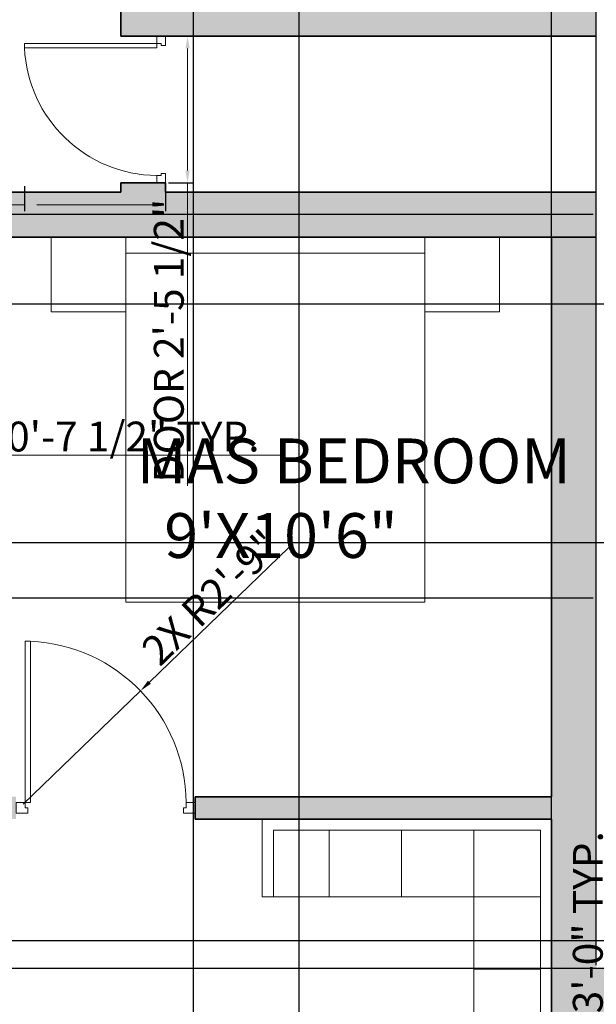
# Model space of a CAD drawing. Units: inches. Extents: x 2696 to 3240, y 1564 to 2310.
# Tile 52 of 76: x 2850 to 2966, y 1982 to 2180. Entities that reach past the tile are written whole.
import ezdxf

# ---------------------------------------------------------------- set-up
doc = ezdxf.new("R2010")
doc.units = ezdxf.units.IN
doc.linetypes.add('ACAD_ISO02W100', pattern=[15, 12, -3])
for name, color, linetype, lineweight in [('A-ANNO-DIMS', 3, 'Continuous', 18), ('A-AREA-IDEN', 7, 'Continuous', 18), ('A-DOOR', 4, 'Continuous', 18), ('A-FURN', 251, 'Continuous', 13), ('A-WALL', 7, 'Continuous', 35), ('A-WALL-OVHD', 7, 'ACAD_ISO02W100', 18), ('A-WALL-PATT', 9, 'Continuous', 13)]:
    doc.layers.add(name, color=color, linetype=linetype, lineweight=lineweight)
doc.styles.add('TIMES NEW', font='times.ttf')
doc.styles.add('YQ_DIM', font='SUPEROS.SHX', dxfattribs={"width": 0.8, "bigfont": 'HZDX.SHX'})
doc.dimstyles.new('Siddhuu', dxfattribs={"dimtxt": 6, "dimasz": 2.5, "dimexe": 1.25, "dimexo": 0.625, "dimtad": 1, "dimdec": 1, "dimlunit": 4, "dimtxsty": 'TIMES NEW', "dimcen": 2.5, "dimclrd": 256, "dimclre": 1, "dimclrt": 7, "dimadec": 0, "dimazin": 0, "dimtfac": 1, "dimtdec": 1, "dimtmove": 0, "dimatfit": 3, "dimfxl": 1, "dimtolj": 1, "dimlwd": -1, "dimarcsym": 0})

# ---------------------------------------------------------------- blocks, each defined once
blk = doc.blocks.new('DR_D01')
for p, q in [((-0.45, 0.93), (-0.42, 0.93)), ((-0.45, 0.03), (-0.45, 0.93)), ((-0.42, 0.03), (-0.42, 0.93)), ((-0.5, 0.03), (-0.42, 0.03)), ((-0.5, 0.03), (-0.5, -0.03)), ((-0.45, 0.03), (-0.45, 0)), ((-0.45, 0), (-0.435, 0)), ((-0.435, 0), (-0.435, -0.03)), ((0.435, 0), (0.435, -0.03)), ((0.45, 0), (0.435, 0)), ((0.45, 0.03), (0.45, 0)), ((0.5, 0.03), (0.45, 0.03)), ((0.5, -0.03), (0.5, 0.03)), ((-0.435, -0.03), (-0.5, -0.03)), ((0.435, -0.03), (0.5, -0.03))]:
    blk.add_line(p, q)
blk.add_arc((-0.4602, 0.0206), 0.9103, 0.5915, 87.4664)
blk = doc.blocks.new('BED-DOUBLE-WITH-NIGHTSTANDS')
for points in [[(0, 75.13), (0, 90.16), (15.03, 90.16), (15.03, 75.13)], [(3.28, 15.03), (3.28, 75.13), (73.4, 75.13), (73.4, 15.03)], [(0, 15.03), (0, 0), (15.03, 0), (15.03, 15.03)]]:
    blk.add_lwpolyline(points, close=True)
blk = doc.blocks.new('SOFA-SECTIONAL')
for p, q in [((0, 43.61), (0, 59.26)), ((0, 59.26), (58.14, 59.26)), ((58.14, 59.26), (58.14, 0)), ((2.24, 43.61), (2.24, 57.02)), ((2.24, 57.02), (55.9, 57.02)), ((13.42, 57.02), (13.42, 43.61)), ((27.95, 57.02), (27.95, 43.61)), ((42.49, 57.02), (42.49, 0)), ((55.9, 57.02), (55.9, 2.24)), ((0, 43.61), (55.9, 43.61)), ((42.49, 29.07), (55.9, 29.07)), ((42.49, 14.54), (55.9, 14.54)), ((55.9, 2.24), (42.49, 2.24)), ((58.14, 0), (42.49, 0))]:
    blk.add_line(p, q)
blk = doc.blocks.new('*D28')
at = {"layer": 'A-ANNO-DIMS', "color": 1, "lineweight": -2, "transparency": 16777216}
for p, q in [((2879.74, 2176.6), (2884.79, 2176.6)), ((2879.74, 2147.07), (2884.79, 2147.07))]:
    blk.add_line(p, q, dxfattribs=at)
at = {"layer": 'A-ANNO-DIMS', "transparency": 16777216}
for p, q in [((2883.54, 2174.1), (2883.54, 2149.57)), ((2883.54, 2147.07), (2883.54, 2086.19))]:
    blk.add_line(p, q, dxfattribs=at)
for points in [[(2883.12, 2174.1), (2883.96, 2174.1), (2883.54, 2176.6)], [(2883.12, 2149.57), (2883.96, 2149.57), (2883.54, 2147.07)]]:
    blk.add_solid(points, dxfattribs=at)
at = {"layer": 'Defpoints', "color": 0, "transparency": 16777216}
for p in [(2879.11, 2176.6), (2879.11, 2147.07), (2883.54, 2147.07)]:
    blk.add_point(p, dxfattribs=at)
at = {"layer": 'A-ANNO-DIMS', "color": 7, "transparency": 16777216, "insert": (2879.77, 2115.38), "char_height": 6, "attachment_point": 5, "rotation": 90, "style": 'TIMES NEW'}
blk.add_mtext('\\A1;DOOR 2\'-5 1/2"', dxfattribs=at)
blk = doc.blocks.new('*D29')
at = {"layer": 'A-ANNO-DIMS', "color": 1, "lineweight": -2, "transparency": 16777216}
for p, q in [((2850.76, 2146.45), (2850.76, 2141.39)), ((2879.11, 2146.45), (2879.11, 2141.39))]:
    blk.add_line(p, q, dxfattribs=at)
at = {"layer": 'A-ANNO-DIMS', "transparency": 16777216}
for p, q in [((2850.76, 2142.64), (2817.24, 2142.64)), ((2876.61, 2142.64), (2853.26, 2142.64))]:
    blk.add_line(p, q, dxfattribs=at)
for points in [[(2853.26, 2143.06), (2853.26, 2142.23), (2850.76, 2142.64)], [(2876.61, 2143.06), (2876.61, 2142.23), (2879.11, 2142.64)]]:
    blk.add_solid(points, dxfattribs=at)
at = {"layer": 'Defpoints', "color": 0, "transparency": 16777216}
for p in [(2850.76, 2147.07), (2879.11, 2147.07), (2850.76, 2142.64)]:
    blk.add_point(p, dxfattribs=at)
at = {"layer": 'A-ANNO-DIMS', "color": 7, "transparency": 16777216, "insert": (2832.75, 2146.41), "char_height": 6, "attachment_point": 5, "style": 'TIMES NEW'}
blk.add_mtext('\\A1;2\'-4 1/2"', dxfattribs=at)
blk = doc.blocks.new('*D30')
at = {"layer": 'A-ANNO-DIMS', "transparency": 16777216}
for p, q in [((2967.69, 1950.58), (2967.69, 2019.05)), ((2967.69, 1917.08), (2967.69, 1948.08))]:
    blk.add_line(p, q, dxfattribs=at)
at = {"layer": 'A-ANNO-DIMS', "color": 1, "lineweight": -2, "transparency": 16777216}
for p, q in [((2962.91, 1950.58), (2968.94, 1950.58)), ((2962.91, 1914.58), (2968.94, 1914.58))]:
    blk.add_line(p, q, dxfattribs=at)
at = {"layer": 'A-ANNO-DIMS', "transparency": 16777216}
for points in [[(2967.27, 1948.08), (2968.11, 1948.08), (2967.69, 1950.58)], [(2967.27, 1917.08), (2968.11, 1917.08), (2967.69, 1914.58)]]:
    blk.add_solid(points, dxfattribs=at)
at = {"layer": 'Defpoints', "color": 0, "transparency": 16777216}
for p in [(2962.29, 1950.58), (2967.69, 1950.58), (2962.29, 1914.58)]:
    blk.add_point(p, dxfattribs=at)
at = {"layer": 'A-ANNO-DIMS', "color": 7, "transparency": 16777216, "insert": (2964, 1986.06), "char_height": 6, "attachment_point": 5, "rotation": 90, "style": 'TIMES NEW'}
blk.add_mtext('\\A1;DOOR 3\'-0" TYP.', dxfattribs=at)
blk = doc.blocks.new('*D40')
at = {"layer": 'A-ANNO-DIMS', "color": 1, "lineweight": -2, "transparency": 16777216}
for p, q in [((2777.27, 2091.83), (2777.27, 2093.58)), ((2784.76, 2091.83), (2784.76, 2093.58))]:
    blk.add_line(p, q, dxfattribs=at)
at = {"layer": 'A-ANNO-DIMS', "transparency": 16777216}
for p, q in [((2779.77, 2092.33), (2782.26, 2092.33)), ((2784.76, 2092.33), (2902.46, 2092.33))]:
    blk.add_line(p, q, dxfattribs=at)
for points in [[(2779.77, 2092.74), (2779.77, 2091.91), (2777.27, 2092.33)], [(2782.26, 2092.74), (2782.26, 2091.91), (2784.76, 2092.33)]]:
    blk.add_solid(points, dxfattribs=at)
at = {"layer": 'Defpoints', "color": 0, "transparency": 16777216}
for p in [(2784.76, 2092.33), (2777.27, 2091.2), (2784.76, 2091.2)]:
    blk.add_point(p, dxfattribs=at)
at = {"layer": 'A-ANNO-DIMS', "color": 7, "transparency": 16777216, "insert": (2844.86, 2096.09), "char_height": 6, "attachment_point": 5, "style": 'TIMES NEW'}
blk.add_mtext('\\A1;BATH FITTING 0\'-7 1/2" TYP.', dxfattribs=at)
blk = doc.blocks.new('*D57')
at = {"layer": 'A-ANNO-DIMS', "color": 1, "lineweight": -2, "transparency": 16777216}
for p, q in [((2754.61, 2018.58), (2754.61, 1568.95)), ((2956.71, 2018.58), (2956.71, 1568.95))]:
    blk.add_line(p, q, dxfattribs=at)
at = {"layer": 'A-ANNO-DIMS', "transparency": 16777216}
blk.add_line((2757.11, 1570.2), (2954.21, 1570.2), dxfattribs=at)
for points in [[(2757.11, 1570.62), (2757.11, 1569.78), (2754.61, 1570.2)], [(2954.21, 1570.62), (2954.21, 1569.78), (2956.71, 1570.2)]]:
    blk.add_solid(points, dxfattribs=at)
at = {"layer": 'Defpoints', "color": 0, "transparency": 16777216}
for p in [(2754.61, 2019.2), (2956.71, 2019.2), (2956.71, 1570.2)]:
    blk.add_point(p, dxfattribs=at)
at = {"layer": 'A-ANNO-DIMS', "color": 7, "transparency": 16777216, "insert": (2855.66, 1573.88), "char_height": 6, "attachment_point": 5, "style": 'TIMES NEW'}
blk.add_mtext('\\A1;16\'-10"', dxfattribs=at)
blk = doc.blocks.new('*D59')
at = {"layer": 'A-ANNO-DIMS', "color": 1, "lineweight": -2, "transparency": 16777216}
for p, q in [((2884.71, 1740.83), (2884.71, 2298.45)), ((2956.71, 1740.83), (2956.71, 2298.45))]:
    blk.add_line(p, q, dxfattribs=at)
at = {"layer": 'A-ANNO-DIMS', "transparency": 16777216}
blk.add_line((2887.21, 2297.2), (2954.21, 2297.2), dxfattribs=at)
for points in [[(2887.21, 2297.62), (2887.21, 2296.78), (2884.71, 2297.2)], [(2954.21, 2297.62), (2954.21, 2296.78), (2956.71, 2297.2)]]:
    blk.add_solid(points, dxfattribs=at)
at = {"layer": 'Defpoints', "color": 0, "transparency": 16777216}
for p in [(2956.71, 2297.2), (2884.71, 1740.2), (2956.71, 1740.2)]:
    blk.add_point(p, dxfattribs=at)
at = {"layer": 'A-ANNO-DIMS', "color": 7, "transparency": 16777216, "insert": (2920.71, 2300.88), "char_height": 6, "attachment_point": 5, "style": 'TIMES NEW'}
blk.add_mtext('\\A1;6\'-0"', dxfattribs=at)
blk = doc.blocks.new('*D61')
at = {"layer": 'A-ANNO-DIMS', "color": 1, "lineweight": -2, "transparency": 16777216}
for p, q in [((2965.71, 2141.33), (2965.71, 2298.45)), ((3044.3, 2141.33), (3044.3, 2298.45))]:
    blk.add_line(p, q, dxfattribs=at)
at = {"layer": 'A-ANNO-DIMS', "transparency": 16777216}
blk.add_line((2968.21, 2297.2), (3041.8, 2297.2), dxfattribs=at)
for points in [[(2968.21, 2297.62), (2968.21, 2296.78), (2965.71, 2297.2)], [(3041.8, 2297.62), (3041.8, 2296.78), (3044.3, 2297.2)]]:
    blk.add_solid(points, dxfattribs=at)
at = {"layer": 'Defpoints', "color": 0, "transparency": 16777216}
for p in [(3044.3, 2297.2), (2965.71, 2140.7), (3044.3, 2140.7)]:
    blk.add_point(p, dxfattribs=at)
at = {"layer": 'A-ANNO-DIMS', "color": 7, "transparency": 16777216, "insert": (3005.01, 2300.96), "char_height": 6, "attachment_point": 5, "style": 'TIMES NEW'}
blk.add_mtext('\\A1;6\'-6 1/2"', dxfattribs=at)
blk = doc.blocks.new('*D62')
at = {"layer": 'A-ANNO-DIMS', "color": 1, "lineweight": -2, "transparency": 16777216}
for p, q in [((2965.08, 2140.7), (2709.36, 2140.7)), ((2965.08, 2063.59), (2709.36, 2063.59))]:
    blk.add_line(p, q, dxfattribs=at)
at = {"layer": 'A-ANNO-DIMS', "transparency": 16777216}
blk.add_line((2710.61, 2066.09), (2710.61, 2138.2), dxfattribs=at)
for points in [[(2710.19, 2138.2), (2711.03, 2138.2), (2710.61, 2140.7)], [(2710.19, 2066.09), (2711.03, 2066.09), (2710.61, 2063.59)]]:
    blk.add_solid(points, dxfattribs=at)
at = {"layer": 'Defpoints', "color": 0, "transparency": 16777216}
for p in [(2710.61, 2140.7), (2965.71, 2140.7), (2965.71, 2063.59)]:
    blk.add_point(p, dxfattribs=at)
at = {"layer": 'A-ANNO-DIMS', "color": 7, "transparency": 16777216, "insert": (2706.93, 2102.15), "char_height": 6, "attachment_point": 5, "rotation": 90, "style": 'TIMES NEW'}
blk.add_mtext('\\A1;6\'-5"', dxfattribs=at)
blk = doc.blocks.new('*D63')
at = {"layer": 'A-ANNO-DIMS', "color": 1, "lineweight": -2, "transparency": 16777216}
for p, q in [((2965.71, 1989.83), (2965.71, 2298.45)), ((3069.21, 1989.83), (3069.21, 2298.45))]:
    blk.add_line(p, q, dxfattribs=at)
at = {"layer": 'A-ANNO-DIMS', "transparency": 16777216}
blk.add_line((2968.21, 2297.2), (3066.71, 2297.2), dxfattribs=at)
for points in [[(2968.21, 2297.62), (2968.21, 2296.78), (2965.71, 2297.2)], [(3066.71, 2297.62), (3066.71, 2296.78), (3069.21, 2297.2)]]:
    blk.add_solid(points, dxfattribs=at)
at = {"layer": 'Defpoints', "color": 0, "transparency": 16777216}
for p in [(3069.21, 2297.2), (2965.71, 1989.2), (3069.21, 1989.2)]:
    blk.add_point(p, dxfattribs=at)
at = {"layer": 'A-ANNO-DIMS', "color": 7, "transparency": 16777216, "insert": (3017.46, 2300.96), "char_height": 6, "attachment_point": 5, "style": 'TIMES NEW'}
blk.add_mtext('\\A1;8\'-7 1/2"', dxfattribs=at)
blk = doc.blocks.new('*D64')
at = {"layer": 'A-ANNO-DIMS', "color": 1, "lineweight": -2, "transparency": 16777216}
for p, q in [((3073.08, 2206.7), (2709.36, 2206.7)), ((3068.58, 1989.2), (2709.36, 1989.2))]:
    blk.add_line(p, q, dxfattribs=at)
at = {"layer": 'A-ANNO-DIMS', "transparency": 16777216}
blk.add_line((2710.61, 1991.7), (2710.61, 2204.2), dxfattribs=at)
for points in [[(2710.19, 2204.2), (2711.03, 2204.2), (2710.61, 2206.7)], [(2710.19, 1991.7), (2711.03, 1991.7), (2710.61, 1989.2)]]:
    blk.add_solid(points, dxfattribs=at)
at = {"layer": 'Defpoints', "color": 0, "transparency": 16777216}
for p in [(2710.61, 2206.7), (3073.71, 2206.7), (3069.21, 1989.2)]:
    blk.add_point(p, dxfattribs=at)
at = {"layer": 'A-ANNO-DIMS', "color": 7, "transparency": 16777216, "insert": (2706.85, 2097.95), "char_height": 6, "attachment_point": 5, "rotation": 90, "style": 'TIMES NEW'}
blk.add_mtext('\\A1;18\'-1 1/2"', dxfattribs=at)
blk = doc.blocks.new('*D66')
at = {"layer": 'A-ANNO-DIMS', "color": 1, "lineweight": -2, "transparency": 16777216}
for p, q in [((3077.58, 2122.7), (2709.36, 2122.7)), ((3077.58, 2074.7), (2709.36, 2074.7))]:
    blk.add_line(p, q, dxfattribs=at)
at = {"layer": 'A-ANNO-DIMS', "transparency": 16777216}
blk.add_line((2710.61, 2077.2), (2710.61, 2120.2), dxfattribs=at)
for points in [[(2710.19, 2120.2), (2711.03, 2120.2), (2710.61, 2122.7)], [(2710.19, 2077.2), (2711.03, 2077.2), (2710.61, 2074.7)]]:
    blk.add_solid(points, dxfattribs=at)
at = {"layer": 'Defpoints', "color": 0, "transparency": 16777216}
for p in [(2710.61, 2122.7), (3078.21, 2122.7), (3078.21, 2074.7)]:
    blk.add_point(p, dxfattribs=at)
at = {"layer": 'A-ANNO-DIMS', "color": 7, "transparency": 16777216, "insert": (2706.93, 2098.7), "char_height": 6, "attachment_point": 5, "rotation": 90, "style": 'TIMES NEW'}
blk.add_mtext('\\A1;4\'-0"', dxfattribs=at)
blk = doc.blocks.new('*D69')
at = {"layer": 'A-ANNO-DIMS', "color": 1, "lineweight": -2, "transparency": 16777216}
for p, q in [((2841.89, 2261.58), (2841.89, 1568.95)), ((2905.91, 2261.58), (2905.91, 1568.95))]:
    blk.add_line(p, q, dxfattribs=at)
at = {"layer": 'A-ANNO-DIMS', "transparency": 16777216}
blk.add_line((2844.39, 1570.2), (2903.41, 1570.2), dxfattribs=at)
for points in [[(2844.39, 1570.62), (2844.39, 1569.78), (2841.89, 1570.2)], [(2903.41, 1570.62), (2903.41, 1569.78), (2905.91, 1570.2)]]:
    blk.add_solid(points, dxfattribs=at)
at = {"layer": 'Defpoints', "color": 0, "transparency": 16777216}
for p in [(2841.89, 2262.2), (2905.91, 2262.2), (2905.91, 1570.2)]:
    blk.add_point(p, dxfattribs=at)
at = {"layer": 'A-ANNO-DIMS', "color": 7, "transparency": 16777216, "insert": (2873.9, 1573.88), "char_height": 6, "attachment_point": 5, "style": 'TIMES NEW'}
blk.add_mtext('\\A1;5\'-4"', dxfattribs=at)
blk = doc.blocks.new('*D77')
at = {"layer": 'A-ANNO-DIMS', "transparency": 16777216}
for p, q in [((2710.61, 1997.2), (2710.61, 2030.6)), ((2710.61, 1989.2), (2710.61, 1994.7)), ((2710.61, 1986.7), (2710.61, 1984.2))]:
    blk.add_line(p, q, dxfattribs=at)
at = {"layer": 'A-ANNO-DIMS', "color": 1, "lineweight": -2, "transparency": 16777216}
for p, q in [((3189.99, 1994.7), (2709.36, 1994.7)), ((3189.99, 1989.2), (2709.36, 1989.2))]:
    blk.add_line(p, q, dxfattribs=at)
at = {"layer": 'A-ANNO-DIMS', "transparency": 16777216}
for points in [[(2710.19, 1997.2), (2711.03, 1997.2), (2710.61, 1994.7)], [(2710.19, 1986.7), (2711.03, 1986.7), (2710.61, 1989.2)]]:
    blk.add_solid(points, dxfattribs=at)
at = {"layer": 'Defpoints', "color": 0, "transparency": 16777216}
for p in [(2710.61, 1994.7), (3190.61, 1994.7), (3190.61, 1989.2)]:
    blk.add_point(p, dxfattribs=at)
at = {"layer": 'A-ANNO-DIMS', "color": 7, "transparency": 16777216, "insert": (2706.85, 2015.15), "char_height": 6, "attachment_point": 5, "rotation": 90, "style": 'TIMES NEW'}
blk.add_mtext('\\A1;0\'-5 1/2"', dxfattribs=at)
blk = doc.blocks.new('*D83')
at = {"layer": 'A-ANNO-DIMS', "transparency": 16777216}
for p, q in [((2903.87, 2073.77), (2875.87, 2046.71)), ((2850.51, 2022.19), (2874.08, 2044.97))]:
    blk.add_line(p, q, dxfattribs=at)
blk.add_solid([(2875.58, 2047.01), (2876.16, 2046.41), (2874.08, 2044.97)], dxfattribs=at)
at = {"layer": 'Defpoints', "color": 0, "transparency": 16777216}
for p in [(2874.08, 2044.97), (2850.51, 2022.19)]:
    blk.add_point(p, dxfattribs=at)
at = {"layer": 'A-ANNO-DIMS', "color": 7, "transparency": 16777216, "insert": (2888.21, 2063.76), "char_height": 6, "attachment_point": 5, "rotation": 44.0287, "style": 'TIMES NEW'}
blk.add_mtext('\\A1;2X R2\'-9"', dxfattribs=at)

msp = doc.modelspace()

# ---------------------------------------------------------------- hatches: boundary and pattern name
at = {"layer": 'A-WALL-PATT', "transparency": 33554556}
h = msp.add_hatch(color=256, dxfattribs=at)
h.dxf.hatch_style = 1
h.paths.add_polyline_path([(2879.11, 2253.2), (2905.91, 2253.2), (2905.91, 2262.2), (2841.89, 2262.2), (2841.89, 2253.2), (2870.11, 2253.2), (2870.11, 2176.6), (2965.71, 2176.6), (2965.71, 2206.7), (2973.58, 2206.7), (2973.58, 2215.7), (2965.71, 2215.7), (2965.71, 2262.2), (2929.91, 2262.2), (2929.91, 2253.2), (2956.71, 2253.2), (2956.71, 2185.6), (2879.11, 2185.6)])
h.paths.add_polyline_path([(2782.83, 2262.2), (2745.61, 2262.2), (2745.61, 2228.73), (2754.61, 2228.73), (2754.61, 2253.2), (2782.83, 2253.2)])
h.paths.add_polyline_path([(2754.61, 2136.2), (2965.71, 2136.2), (2965.71, 2145.2), (2879.11, 2145.2), (2879.11, 2147.07), (2877.34, 2147.07), (2870.11, 2147.07), (2870.11, 2145.2), (2754.61, 2145.2), (2754.61, 2169.67), (2745.61, 2169.67), (2745.61, 2000.2), (2754.61, 2000.2), (2754.61, 2019.2), (2849.08, 2019.2), (2849.08, 2023.7), (2841.21, 2023.7), (2841.21, 2051.83), (2836.71, 2051.83), (2836.71, 2023.7), (2754.61, 2023.7), (2754.61, 2091.2), (2836.71, 2091.2), (2836.71, 2087.83), (2841.21, 2087.83), (2841.21, 2095.7), (2754.61, 2095.7)])
h.paths.add_polyline_path([(2965.71, 2136.2), (2956.71, 2136.2), (2956.71, 2023.7), (2885.08, 2023.7), (2885.08, 2019.2), (2956.71, 2019.2), (2956.71, 1950.58), (2965.71, 1950.58), (2965.71, 1980.2), (2973.58, 1980.2), (2973.58, 1989.2), (2965.71, 1989.2)])
h.paths.add_polyline_path([(2754.61, 1906.7), (2880.21, 1906.7), (2884.71, 1906.7), (2956.71, 1906.7), (2956.71, 1792.7), (2944.71, 1792.7), (2944.71, 1783.7), (2956.71, 1783.7), (2956.71, 1740.2), (2884.71, 1740.2), (2884.71, 1783.7), (2896.71, 1783.7), (2896.71, 1792.7), (2884.71, 1792.7), (2884.71, 1846.7), (2880.21, 1846.7), (2880.21, 1740.2), (2754.61, 1740.2), (2754.61, 1777.2), (2745.61, 1777.2), (2745.61, 1692.7), (2754.61, 1692.7), (2754.61, 1731.2), (2956.71, 1731.2), (2956.71, 1723.33), (2965.71, 1723.33), (2965.71, 1884.2), (2973.58, 1884.2), (2973.58, 1893.2), (2965.71, 1893.2), (2965.71, 1914.58), (2956.71, 1914.58), (2956.71, 1911.2), (2754.61, 1911.2), (2754.61, 1930.2), (2745.61, 1930.2), (2745.61, 1817.2), (2754.61, 1817.2), (2754.61, 1854.2), (2826.61, 1854.2), (2826.61, 1868.83), (2822.11, 1868.83), (2822.11, 1858.7), (2754.61, 1858.7)])
h.paths.add_polyline_path([(2965.71, 1656.2), (3008.24, 1656.2), (3008.24, 1665.2), (2965.71, 1665.2), (2965.71, 1693.33), (2956.71, 1693.33), (2956.71, 1686.2), (2934.58, 1686.2), (2934.58, 1681.7), (2956.71, 1681.7), (2956.71, 1614.2), (2896.71, 1614.2), (2896.71, 1681.7), (2904.58, 1681.7), (2904.58, 1686.2), (2892.21, 1686.2), (2892.21, 1614.2), (2858.41, 1614.2), (2858.41, 1605.2), (2965.71, 1605.2)])
h.paths.add_polyline_path([(2788.41, 1614.2), (2754.61, 1614.2), (2754.61, 1652.7), (2745.61, 1652.7), (2745.61, 1605.2), (2788.41, 1605.2)])
h.paths.add_polyline_path([(3199.61, 1633.05), (3190.61, 1633.05), (3190.61, 1614.2), (3082.61, 1614.2), (3082.61, 1665.2), (3070.24, 1665.2), (3070.24, 1656.2), (3078.11, 1656.2), (3078.11, 1605.2), (3199.61, 1605.2)])
h.paths.add_polyline_path([(3199.61, 1702.05), (3190.61, 1702.05), (3190.61, 1699.7), (3106.61, 1699.7), (3106.61, 1747.7), (3190.61, 1747.7), (3190.61, 1752.2), (3082.61, 1752.2), (3082.61, 1760.08), (3078.11, 1760.08), (3078.11, 1747.7), (3102.11, 1747.7), (3102.11, 1699.7), (3078.11, 1699.7), (3078.11, 1695.2), (3190.61, 1695.2), (3190.61, 1676.35), (3199.61, 1676.35)])
h.paths.add_polyline_path([(3199.61, 1783.2), (3190.61, 1783.2), (3190.61, 1745.35), (3199.61, 1745.35)])
h.paths.add_polyline_path([(3082.61, 1884.2), (3190.61, 1884.2), (3190.61, 1853.2), (3199.61, 1853.2), (3199.61, 1901.7), (3190.61, 1901.7), (3190.61, 1893.2), (3005.58, 1893.2), (3005.58, 1891.28), (3005.58, 1884.2), (3078.11, 1884.2), (3078.11, 1792.08), (3082.61, 1792.08)])
h.paths.add_polyline_path([(3199.61, 1994.7), (3190.61, 1994.7), (3190.61, 1989.2), (3073.71, 1989.2), (3073.71, 2034.2), (3069.21, 2034.2), (3069.21, 1989.2), (3005.58, 1989.2), (3005.58, 1980.2), (3190.61, 1980.2), (3190.61, 1971.7), (3199.61, 1971.7)])
h.paths.add_polyline_path([(3199.61, 2155.2), (3190.61, 2155.2), (3190.61, 2064.7), (3199.61, 2064.7)])
h.paths.add_polyline_path([(3190.61, 2074.7), (3106.61, 2074.7), (3106.61, 2122.7), (3190.61, 2122.7), (3190.61, 2127.2), (3082.71, 2127.2), (3082.71, 2135.08), (3073.71, 2135.08), (3073.71, 2122.7), (3102.11, 2122.7), (3102.11, 2074.7), (3069.21, 2074.7), (3069.21, 2070.2), (3190.61, 2070.2)])
h.paths.add_polyline_path([(3082.71, 2253.2), (3190.61, 2253.2), (3190.61, 2225.2), (3199.61, 2225.2), (3199.61, 2262.2), (3073.71, 2262.2), (3073.71, 2215.7), (3035.58, 2215.7), (3035.58, 2206.7), (3073.71, 2206.7), (3073.71, 2171.08), (3082.71, 2171.08)])

# ---------------------------------------------------------------- linework, layer by layer
at = {"layer": 'A-WALL'}
for p, q in [((2870.11, 2176.6), (2870.11, 2253.2)), ((2870.11, 2176.6), (2965.71, 2176.6)), ((2870.11, 2147.07), (2870.11, 2145.2)), ((2879.11, 2147.07), (2870.11, 2147.07)), ((2879.11, 2147.07), (2879.11, 2145.2)), ((2754.61, 2145.2), (2870.11, 2145.2)), ((2879.11, 2145.2), (2965.71, 2145.2)), ((2754.61, 2136.2), (2965.71, 2136.2)), ((2956.71, 2136.2), (2956.71, 2023.7)), ((2885.08, 2023.7), (2956.71, 2023.7)), ((2885.08, 2023.7), (2885.08, 2019.2)), ((2885.08, 2019.2), (2956.71, 2019.2)), ((2956.71, 2019.2), (2956.71, 1950.58))]:
    msp.add_line(p, q, dxfattribs=at)
at = {"layer": 'A-WALL-OVHD'}
msp.add_line((2956.71, 2176.6), (2956.71, 2145.2), dxfattribs=at)

# ---------------------------------------------------------------- block references
at = {"layer": 'A-DOOR', "xscale": 29.52755905511811, "yscale": -29.52755905511811, "zscale": 29.52755905511811, "rotation": 270}
msp.add_blockref('DR_D01', (2878.23, 2161.84), dxfattribs=at)
at = {"layer": 'A-DOOR', "xscale": 36, "yscale": 36, "zscale": 36}
msp.add_blockref('DR_D01', (2867.08, 2021.45), dxfattribs=at)
at = {"layer": 'A-FURN', "rotation": 269.9999999999998}
msp.add_blockref('BED-DOUBLE-WITH-NIGHTSTANDS', (2856.1, 2136.2), dxfattribs=at)
at = {"layer": 'A-FURN'}
msp.add_blockref('SOFA-SECTIONAL', (2898.57, 1959.94), dxfattribs=at)

# ---------------------------------------------------------------- texts
at = {"layer": 'A-AREA-IDEN', "insert": (2873.36, 2095.7), "char_height": 9, "attachment_point": 1, "style": 'YQ_DIM'}
msp.add_mtext_dynamic_manual_height_columns('MAS BEDROOM\\P  9\'X10\'6"', width=92.6128, gutter_width=12.5, heights=[0], dxfattribs=at)

# ---------------------------------------------------------------- dimensions: what is measured, and where the dimension line sits
at = {"layer": 'A-ANNO-DIMS'}
for base, p1, p2, picture, middle in [((3044.3, 2297.2), (2965.71, 2140.7), (3044.3, 2140.7), '*D61', (3005.01, 2300.96)), ((3069.21, 2297.2), (2965.71, 1989.2), (3069.21, 1989.2), '*D63', (3017.46, 2300.96)), ((2956.71, 2297.2), (2884.71, 1740.2), (2956.71, 1740.2), '*D59', (2920.71, 2300.88)), ((2905.91, 1570.2), (2841.89, 2262.2), (2905.91, 2262.2), '*D69', (2873.9, 1573.88)), ((2956.71, 1570.2), (2754.61, 2019.2), (2956.71, 2019.2), '*D57', (2855.66, 1573.88))]:
    dim = msp.add_linear_dim(base=base, p1=p1, p2=p2, dimstyle='Siddhuu', override={"dimdec": 1, "dimlfac": 1, "dimrnd": 0, "dimzin": 1, "dimdsep": 46, "dimlunit": 4, "dimfrac": 2}, dxfattribs=at)
    dim.commit()
    dim.dimension.update_dxf_attribs({"geometry": picture, "text_midpoint": middle})
for base, p1, p2, angle, picture, middle in [((2710.61, 2206.7), (3069.21, 1989.2), (3073.71, 2206.7), 90, '*D64', (2706.85, 2097.95)), ((2850.7649, 2142.6444), (2879.1114, 2147.0735), (2850.7649, 2147.0735), 180, '*D29', (2832.7503, 2146.4057)), ((2710.61, 2140.7), (2965.71, 2063.59), (2965.71, 2140.7), 90, '*D62', (2706.93, 2102.15)), ((2710.61, 2122.7), (3078.21, 2074.7), (3078.21, 2122.7), 90, '*D66', (2706.93, 2098.7)), ((2710.61, 1994.7), (3190.61, 1989.2), (3190.61, 1994.7), 90, '*D77', (2706.85, 2015.15))]:
    dim = msp.add_linear_dim(base=base, p1=p1, p2=p2, angle=angle, dimstyle='Siddhuu', override={"dimdec": 1, "dimlfac": 1, "dimrnd": 0, "dimzin": 1, "dimdsep": 46, "dimlunit": 4, "dimfrac": 2}, dxfattribs=at)
    dim.commit()
    dim.dimension.update_dxf_attribs({"geometry": picture, "text_midpoint": middle})
for base, p1, p2, angle, text, picture, middle in [((2883.54, 2147.07), (2879.11, 2176.6), (2879.11, 2147.07), 270, 'DOOR <>', '*D28', (2879.77, 2115.38)), ((2967.69, 1950.58), (2962.29, 1914.58), (2962.29, 1950.58), 90, 'DOOR <> TYP.', '*D30', (2964, 1986.06))]:
    dim = msp.add_linear_dim(base=base, p1=p1, p2=p2, angle=angle, text=text, dimstyle='Siddhuu', override={"dimdec": 1, "dimlfac": 1, "dimrnd": 0, "dimzin": 1, "dimdsep": 46, "dimlunit": 4, "dimfrac": 2}, dxfattribs=at)
    dim.commit()
    dim.dimension.update_dxf_attribs({"geometry": picture, "text_midpoint": middle})
dim = msp.add_linear_dim(base=(2784.76, 2092.33), p1=(2777.27, 2091.2), p2=(2784.76, 2091.2), text='BATH FITTING <> TYP.', dimstyle='Siddhuu', override={"dimdec": 1, "dimlfac": 1, "dimrnd": 0, "dimzin": 1, "dimdsep": 46, "dimlunit": 4, "dimfrac": 2}, dxfattribs=at)
dim.commit()
dim.dimension.update_dxf_attribs({"geometry": '*D40', "text_midpoint": (2844.86, 2096.09)})
dim = msp.add_radius_dim(center=(2850.51, 2022.19), mpoint=(2874.08, 2044.97), text='2X <>', dimstyle='Siddhuu', override={"dimdec": 1, "dimlfac": 1, "dimrnd": 0, "dimzin": 1, "dimdsep": 46, "dimlunit": 4, "dimfrac": 2}, dxfattribs=at)
dim.commit()
dim.dimension.update_dxf_attribs({"geometry": '*D83', "text_midpoint": (2888.21, 2063.76)})

doc.saveas('drawing.dxf')
